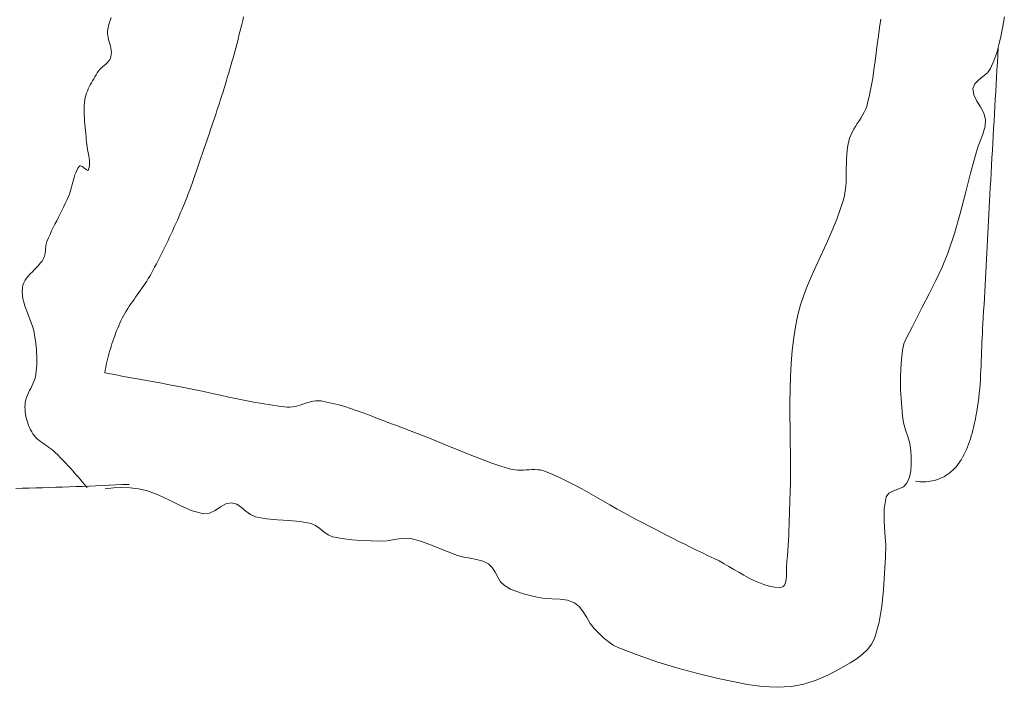
# Model space of a CAD drawing. Units: inches. Extents: x -15 to 423, y -713 to 71.
# Tile 13 of 24: x 333 to 357, y -341 to -324. Entities that reach past the tile are written whole.
import ezdxf

# ---------------------------------------------------------------- set-up
doc = ezdxf.new("R2010")
doc.units = ezdxf.units.IN
doc.header["$MEASUREMENT"] = 0
doc.layers.add('A-FURN', color=9, linetype='Continuous', lineweight=13)

# ---------------------------------------------------------------- blocks, each defined once
blk = doc.blocks.new('BED-DOUBLE')
for p, q in [((72.488, 18.091), (72.461, 18.02)), ((75.772, 18.106), (75.749, 18.013)), ((94.613, 17.825), (94.657, 18.111)), ((72.415, 17.876), (72.399, 17.803)), ((72.436, 17.949), (72.415, 17.876)), ((72.461, 18.02), (72.436, 17.949)), ((75.727, 17.92), (75.704, 17.827)), ((75.749, 18.013), (75.727, 17.92)), ((91.529, 17.634), (91.558, 17.844)), ((91.558, 17.844), (91.59, 18.053)), ((72.399, 17.803), (72.392, 17.751)), ((72.392, 17.751), (72.392, 17.698)), ((72.392, 17.698), (72.398, 17.646)), ((72.398, 17.646), (72.408, 17.593)), ((75.657, 17.642), (75.633, 17.549)), ((75.681, 17.735), (75.657, 17.642)), ((75.704, 17.827), (75.681, 17.735)), ((91.502, 17.424), (91.529, 17.634)), ((94.524, 17.415), (94.571, 17.62)), ((94.571, 17.62), (94.613, 17.825)), ((72.408, 17.593), (72.421, 17.54)), ((72.421, 17.54), (72.435, 17.487)), ((72.435, 17.487), (72.45, 17.434)), ((72.45, 17.434), (72.464, 17.382)), ((72.464, 17.382), (72.476, 17.329)), ((75.584, 17.364), (75.559, 17.272)), ((75.609, 17.457), (75.584, 17.364)), ((75.633, 17.549), (75.609, 17.457)), ((91.476, 17.214), (91.502, 17.424)), ((94.468, 17.212), (94.524, 17.415)), ((72.479, 17.121), (72.467, 17.083)), ((72.476, 17.329), (72.485, 17.276)), ((72.488, 17.172), (72.479, 17.121)), ((72.485, 17.276), (72.489, 17.224)), ((72.489, 17.224), (72.488, 17.172)), ((75.534, 17.179), (75.509, 17.087)), ((75.559, 17.272), (75.534, 17.179)), ((91.449, 17.004), (91.476, 17.214)), ((94.4, 17.014), (94.468, 17.212)), ((94.483, 16.977), (94.494, 17.16)), ((94.494, 17.16), (94.504, 17.342)), ((72.28, 16.872), (72.248, 16.844)), ((72.312, 16.899), (72.28, 16.872)), ((72.344, 16.927), (72.312, 16.899)), ((72.374, 16.955), (72.344, 16.927)), ((72.402, 16.984), (72.374, 16.955)), ((72.428, 17.015), (72.402, 16.984)), ((72.45, 17.048), (72.428, 17.015)), ((72.467, 17.083), (72.45, 17.048)), ((75.457, 16.903), (75.431, 16.811)), ((75.483, 16.995), (75.457, 16.903)), ((75.509, 17.087), (75.483, 16.995)), ((91.421, 16.794), (91.449, 17.004)), ((94.317, 16.822), (94.4, 17.014)), ((94.473, 16.795), (94.483, 16.977)), ((72.08, 16.623), (72.05, 16.573)), ((72.11, 16.672), (72.08, 16.623)), ((72.139, 16.721), (72.11, 16.672)), ((72.162, 16.754), (72.139, 16.721)), ((72.188, 16.785), (72.162, 16.754)), ((72.217, 16.815), (72.188, 16.785)), ((72.248, 16.844), (72.217, 16.815)), ((75.376, 16.625), (75.348, 16.53)), ((75.404, 16.719), (75.376, 16.625)), ((75.431, 16.811), (75.404, 16.719)), ((91.389, 16.585), (91.421, 16.794)), ((94.013, 16.539), (94.126, 16.626)), ((94.126, 16.626), (94.236, 16.716)), ((94.236, 16.716), (94.317, 16.822)), ((94.463, 16.612), (94.473, 16.795)), ((71.965, 16.422), (71.94, 16.371)), ((71.993, 16.473), (71.965, 16.422)), ((72.021, 16.523), (71.993, 16.473)), ((72.05, 16.573), (72.021, 16.523)), ((75.32, 16.436), (75.291, 16.342)), ((75.348, 16.53), (75.32, 16.436)), ((91.353, 16.376), (91.389, 16.585)), ((93.877, 16.327), (93.922, 16.444)), ((93.922, 16.444), (94.013, 16.539)), ((94.442, 16.248), (94.452, 16.43)), ((94.452, 16.43), (94.463, 16.612)), ((71.856, 16.159), (71.842, 16.104)), ((71.874, 16.213), (71.856, 16.159)), ((71.893, 16.266), (71.874, 16.213)), ((71.915, 16.319), (71.893, 16.266)), ((71.94, 16.371), (71.915, 16.319)), ((75.232, 16.155), (75.202, 16.061)), ((75.262, 16.248), (75.232, 16.155)), ((75.291, 16.342), (75.262, 16.248)), ((91.264, 15.963), (91.312, 16.169)), ((91.312, 16.169), (91.353, 16.376)), ((93.898, 16.169), (93.877, 16.327)), ((93.971, 16.019), (93.898, 16.169)), ((94.432, 16.065), (94.442, 16.248)), ((71.815, 15.897), (71.812, 15.821)), ((71.821, 15.972), (71.815, 15.897)), ((71.831, 16.048), (71.821, 15.972)), ((71.842, 16.104), (71.831, 16.048)), ((75.172, 15.967), (75.141, 15.874)), ((75.202, 16.061), (75.172, 15.967)), ((91.241, 15.886), (91.264, 15.963)), ((94.065, 15.871), (93.971, 16.019)), ((94.421, 15.883), (94.432, 16.065)), ((71.812, 15.821), (71.812, 15.745)), ((71.812, 15.745), (71.814, 15.668)), ((71.814, 15.668), (71.819, 15.592)), ((75.079, 15.687), (75.048, 15.594)), ((75.11, 15.78), (75.079, 15.687)), ((75.141, 15.874), (75.11, 15.78)), ((91.095, 15.597), (91.137, 15.668)), ((91.137, 15.668), (91.176, 15.739)), ((91.176, 15.739), (91.211, 15.812)), ((91.211, 15.812), (91.241, 15.886)), ((94.149, 15.721), (94.065, 15.871)), ((94.189, 15.562), (94.149, 15.721)), ((94.401, 15.518), (94.411, 15.7)), ((94.411, 15.7), (94.421, 15.883)), ((71.819, 15.592), (71.825, 15.515)), ((71.825, 15.515), (71.832, 15.439)), ((71.832, 15.439), (71.839, 15.362)), ((74.985, 15.407), (74.954, 15.314)), ((75.017, 15.5), (74.985, 15.407)), ((75.048, 15.594), (75.017, 15.5)), ((90.963, 15.389), (91.007, 15.458)), ((91.007, 15.458), (91.051, 15.528)), ((91.051, 15.528), (91.095, 15.597)), ((94.177, 15.392), (94.189, 15.562)), ((94.391, 15.335), (94.401, 15.518)), ((71.839, 15.362), (71.847, 15.285)), ((71.847, 15.285), (71.854, 15.209)), ((71.854, 15.209), (71.86, 15.132)), ((74.922, 15.221), (74.89, 15.128)), ((74.954, 15.314), (74.922, 15.221)), ((90.817, 15.1), (90.847, 15.175)), ((90.847, 15.175), (90.882, 15.247)), ((90.882, 15.247), (90.921, 15.319)), ((90.921, 15.319), (90.963, 15.389)), ((94.075, 15.061), (94.135, 15.225)), ((94.135, 15.225), (94.177, 15.392)), ((94.38, 15.153), (94.391, 15.335)), ((71.86, 15.132), (71.865, 15.056)), ((71.865, 15.056), (71.87, 14.999)), ((71.87, 14.999), (71.877, 14.942)), ((71.877, 14.942), (71.887, 14.884)), ((74.827, 14.942), (74.795, 14.849)), ((74.859, 15.035), (74.827, 14.942)), ((74.89, 15.128), (74.859, 15.035)), ((90.755, 14.802), (90.771, 14.913)), ((90.771, 14.913), (90.794, 15.023)), ((90.794, 15.023), (90.817, 15.1)), ((94.01, 14.897), (94.075, 15.061)), ((94.36, 14.788), (94.37, 14.971)), ((94.37, 14.971), (94.38, 15.153)), ((71.887, 14.884), (71.897, 14.827)), ((71.897, 14.827), (71.908, 14.769)), ((71.908, 14.769), (71.919, 14.712)), ((71.919, 14.712), (71.928, 14.654)), ((74.746, 14.703), (74.721, 14.63)), ((74.77, 14.776), (74.746, 14.703)), ((74.795, 14.849), (74.77, 14.776)), ((90.738, 14.577), (90.744, 14.69)), ((90.744, 14.69), (90.755, 14.802)), ((93.82, 14.232), (93.955, 14.732)), ((93.955, 14.732), (94.01, 14.897)), ((94.35, 14.606), (94.36, 14.788)), ((71.928, 14.654), (71.936, 14.597)), ((71.936, 14.597), (71.942, 14.54)), ((71.943, 14.427), (71.937, 14.371)), ((71.942, 14.54), (71.944, 14.484)), ((71.944, 14.484), (71.943, 14.427)), ((74.672, 14.485), (74.647, 14.412)), ((74.697, 14.557), (74.672, 14.485)), ((74.721, 14.63), (74.697, 14.557)), ((90.734, 14.351), (90.735, 14.464)), ((90.735, 14.464), (90.738, 14.577)), ((94.329, 14.241), (94.34, 14.423)), ((94.34, 14.423), (94.35, 14.606)), ((71.583, 14.184), (71.563, 14.125)), ((71.605, 14.241), (71.583, 14.184)), ((71.63, 14.296), (71.605, 14.241)), ((71.66, 14.349), (71.63, 14.296)), ((71.694, 14.399), (71.66, 14.349)), ((71.707, 14.41), (71.694, 14.399)), ((71.724, 14.411), (71.707, 14.41)), ((71.743, 14.405), (71.724, 14.411)), ((71.764, 14.394), (71.743, 14.405)), ((71.786, 14.379), (71.764, 14.394)), ((71.809, 14.361), (71.786, 14.379)), ((71.831, 14.344), (71.809, 14.361)), ((71.853, 14.327), (71.831, 14.344)), ((71.873, 14.313), (71.853, 14.327)), ((71.891, 14.303), (71.873, 14.313)), ((71.907, 14.299), (71.891, 14.303)), ((71.918, 14.303), (71.907, 14.299)), ((71.925, 14.316), (71.918, 14.303)), ((71.937, 14.371), (71.925, 14.316)), ((74.573, 14.194), (74.547, 14.121)), ((74.598, 14.266), (74.573, 14.194)), ((74.623, 14.339), (74.598, 14.266)), ((74.647, 14.412), (74.623, 14.339)), ((90.732, 14.124), (90.734, 14.237)), ((90.734, 14.237), (90.734, 14.351)), ((93.691, 13.73), (93.82, 14.232)), ((94.319, 14.058), (94.329, 14.241)), ((71.515, 13.945), (71.499, 13.884)), ((71.53, 14.005), (71.515, 13.945)), ((71.546, 14.066), (71.53, 14.005)), ((71.563, 14.125), (71.546, 14.066)), ((74.496, 13.976), (74.47, 13.904)), ((74.522, 14.049), (74.496, 13.976)), ((74.547, 14.121), (74.522, 14.049)), ((90.72, 13.898), (90.728, 14.011)), ((90.728, 14.011), (90.732, 14.124)), ((94.309, 13.876), (94.319, 14.058)), ((71.446, 13.705), (71.423, 13.648)), ((71.465, 13.764), (71.446, 13.705)), ((71.483, 13.824), (71.465, 13.764)), ((71.499, 13.884), (71.483, 13.824)), ((74.389, 13.688), (74.361, 13.617)), ((74.416, 13.76), (74.389, 13.688)), ((74.443, 13.832), (74.416, 13.76)), ((74.47, 13.904), (74.443, 13.832)), ((90.688, 13.677), (90.707, 13.787)), ((90.707, 13.787), (90.72, 13.898)), ((93.559, 13.23), (93.691, 13.73)), ((94.29, 13.533), (94.299, 13.693)), ((94.299, 13.693), (94.309, 13.876)), ((71.344, 13.475), (71.303, 13.389)), ((71.385, 13.561), (71.344, 13.475)), ((71.423, 13.648), (71.385, 13.561)), ((74.304, 13.474), (74.274, 13.404)), ((74.333, 13.546), (74.304, 13.474)), ((74.361, 13.617), (74.333, 13.546)), ((90.584, 13.325), (90.662, 13.568)), ((90.662, 13.568), (90.688, 13.677)), ((94.281, 13.373), (94.29, 13.533)), ((71.218, 13.219), (71.175, 13.135)), ((71.261, 13.304), (71.218, 13.219)), ((71.303, 13.389), (71.261, 13.304)), ((74.201, 13.233), (74.164, 13.148)), ((74.238, 13.318), (74.201, 13.233)), ((74.274, 13.404), (74.238, 13.318)), ((90.497, 13.085), (90.584, 13.325)), ((93.416, 12.733), (93.559, 13.23)), ((94.264, 13.053), (94.273, 13.213)), ((94.273, 13.213), (94.281, 13.373)), ((71.089, 12.965), (71.047, 12.88)), ((71.132, 13.05), (71.089, 12.965)), ((71.175, 13.135), (71.132, 13.05)), ((74.089, 12.979), (74.051, 12.894)), ((74.127, 13.064), (74.089, 12.979)), ((74.164, 13.148), (74.127, 13.064)), ((90.4, 12.848), (90.497, 13.085)), ((94.256, 12.893), (94.264, 13.053)), ((71.006, 12.794), (70.966, 12.708)), ((71.047, 12.88), (71.006, 12.794)), ((73.974, 12.726), (73.935, 12.642)), ((74.013, 12.81), (73.974, 12.726)), ((74.051, 12.894), (74.013, 12.81)), ((90.297, 12.612), (90.4, 12.848)), ((93.253, 12.242), (93.416, 12.733)), ((94.239, 12.572), (94.248, 12.733)), ((94.248, 12.733), (94.256, 12.893)), ((70.871, 12.47), (70.865, 12.437)), ((70.88, 12.502), (70.871, 12.47)), ((70.891, 12.534), (70.88, 12.502)), ((70.927, 12.621), (70.891, 12.534)), ((70.966, 12.708), (70.927, 12.621)), ((73.855, 12.474), (73.815, 12.391)), ((73.895, 12.558), (73.855, 12.474)), ((73.935, 12.642), (73.895, 12.558)), ((90.191, 12.378), (90.297, 12.612)), ((94.231, 12.412), (94.239, 12.572)), ((70.842, 12.235), (70.836, 12.202)), ((70.846, 12.268), (70.842, 12.235)), ((70.85, 12.302), (70.846, 12.268)), ((70.853, 12.336), (70.85, 12.302)), ((70.856, 12.37), (70.853, 12.336)), ((70.86, 12.403), (70.856, 12.37)), ((70.865, 12.437), (70.86, 12.403)), ((73.733, 12.225), (73.691, 12.142)), ((73.774, 12.308), (73.733, 12.225)), ((73.815, 12.391), (73.774, 12.308)), ((90.083, 12.145), (90.191, 12.378)), ((93.115, 11.899), (93.253, 12.242)), ((94.214, 12.092), (94.223, 12.252)), ((94.223, 12.252), (94.231, 12.412)), ((70.725, 11.993), (70.679, 11.939)), ((70.767, 12.049), (70.725, 11.993)), ((70.802, 12.108), (70.767, 12.049)), ((70.816, 12.138), (70.802, 12.108)), ((70.827, 12.17), (70.816, 12.138)), ((70.836, 12.202), (70.827, 12.17)), ((73.606, 11.977), (73.563, 11.895)), ((73.649, 12.06), (73.606, 11.977)), ((73.691, 12.142), (73.649, 12.06)), ((89.975, 11.911), (90.083, 12.145)), ((94.206, 11.932), (94.214, 12.092)), ((70.527, 11.783), (70.477, 11.732)), ((70.578, 11.835), (70.527, 11.783)), ((70.629, 11.886), (70.578, 11.835)), ((70.679, 11.939), (70.629, 11.886)), ((73.519, 11.814), (73.475, 11.732)), ((73.563, 11.895), (73.519, 11.814)), ((89.871, 11.676), (89.975, 11.911)), ((92.957, 11.564), (93.115, 11.899)), ((94.189, 11.612), (94.197, 11.772)), ((94.197, 11.772), (94.206, 11.932)), ((70.316, 11.511), (70.293, 11.449)), ((70.347, 11.57), (70.316, 11.511)), ((70.385, 11.626), (70.347, 11.57)), ((70.429, 11.68), (70.385, 11.626)), ((70.477, 11.732), (70.429, 11.68)), ((73.331, 11.495), (73.293, 11.438)), ((73.369, 11.553), (73.331, 11.495)), ((73.406, 11.612), (73.369, 11.553)), ((73.441, 11.672), (73.406, 11.612)), ((73.475, 11.732), (73.441, 11.672)), ((89.772, 11.441), (89.871, 11.676)), ((92.788, 11.233), (92.957, 11.564)), ((94.18, 11.451), (94.189, 11.612)), ((70.279, 11.383), (70.274, 11.292)), ((70.274, 11.292), (70.28, 11.202)), ((70.293, 11.449), (70.279, 11.383)), ((73.173, 11.267), (73.132, 11.21)), ((73.213, 11.323), (73.173, 11.267)), ((73.253, 11.38), (73.213, 11.323)), ((73.293, 11.438), (73.253, 11.38)), ((89.681, 11.202), (89.772, 11.441)), ((94.162, 11.131), (94.171, 11.291)), ((94.171, 11.291), (94.18, 11.451)), ((70.28, 11.202), (70.294, 11.113)), ((70.294, 11.113), (70.315, 11.025)), ((70.315, 11.025), (70.342, 10.936)), ((73.012, 11.04), (72.972, 10.983)), ((73.052, 11.097), (73.012, 11.04)), ((73.092, 11.153), (73.052, 11.097)), ((73.132, 11.21), (73.092, 11.153)), ((89.6, 10.961), (89.681, 11.202)), ((92.618, 10.903), (92.788, 11.233)), ((94.153, 10.971), (94.162, 11.131)), ((70.342, 10.936), (70.373, 10.849)), ((70.373, 10.849), (70.407, 10.761)), ((70.407, 10.761), (70.442, 10.673)), ((72.859, 10.808), (72.824, 10.749)), ((72.896, 10.867), (72.859, 10.808)), ((72.934, 10.925), (72.896, 10.867)), ((72.972, 10.983), (72.934, 10.925)), ((89.532, 10.717), (89.6, 10.961)), ((92.454, 10.571), (92.618, 10.903)), ((94.134, 10.651), (94.143, 10.811)), ((94.143, 10.811), (94.153, 10.971)), ((70.442, 10.673), (70.477, 10.585)), ((70.477, 10.585), (70.51, 10.497)), ((72.728, 10.565), (72.7, 10.503)), ((72.758, 10.627), (72.728, 10.565)), ((72.79, 10.688), (72.758, 10.627)), ((72.824, 10.749), (72.79, 10.688)), ((89.478, 10.468), (89.532, 10.717)), ((92.38, 10.427), (92.454, 10.571)), ((94.124, 10.491), (94.134, 10.651)), ((70.51, 10.497), (70.539, 10.408)), ((70.539, 10.408), (70.564, 10.319)), ((70.564, 10.319), (70.582, 10.229)), ((72.62, 10.316), (72.595, 10.253)), ((72.646, 10.379), (72.62, 10.316)), ((72.672, 10.441), (72.646, 10.379)), ((72.7, 10.503), (72.672, 10.441)), ((89.428, 10.15), (89.478, 10.468)), ((92.224, 10.142), (92.3, 10.285)), ((92.3, 10.285), (92.38, 10.427)), ((94.111, 10.262), (94.117, 10.376)), ((94.117, 10.376), (94.124, 10.491)), ((70.582, 10.229), (70.593, 10.153)), ((70.593, 10.153), (70.604, 10.077)), ((70.604, 10.077), (70.613, 10.001)), ((72.526, 10.062), (72.504, 9.997)), ((72.548, 10.126), (72.526, 10.062)), ((72.571, 10.19), (72.548, 10.126)), ((72.595, 10.253), (72.571, 10.19)), ((89.39, 9.83), (89.428, 10.15)), ((92.163, 9.994), (92.224, 10.142)), ((94.097, 9.917), (94.101, 10.032)), ((94.101, 10.032), (94.106, 10.147)), ((94.106, 10.147), (94.111, 10.262)), ((70.613, 10.001), (70.621, 9.924)), ((70.621, 9.924), (70.628, 9.848)), ((70.628, 9.848), (70.633, 9.771)), ((72.445, 9.802), (72.427, 9.736)), ((72.464, 9.867), (72.445, 9.802)), ((72.484, 9.932), (72.464, 9.867)), ((72.504, 9.997), (72.484, 9.932)), ((89.363, 9.509), (89.39, 9.83)), ((92.092, 9.515), (92.125, 9.84)), ((92.125, 9.84), (92.163, 9.994)), ((94.089, 9.687), (94.093, 9.802)), ((94.093, 9.802), (94.097, 9.917)), ((70.633, 9.771), (70.636, 9.695)), ((70.636, 9.695), (70.638, 9.618)), ((70.638, 9.541), (70.636, 9.465)), ((70.638, 9.618), (70.638, 9.541)), ((72.379, 9.539), (72.364, 9.472)), ((72.394, 9.605), (72.379, 9.539)), ((72.41, 9.671), (72.394, 9.605)), ((72.427, 9.736), (72.41, 9.671)), ((94.08, 9.457), (94.085, 9.572)), ((94.085, 9.572), (94.089, 9.687)), ((70.625, 9.312), (70.616, 9.236)), ((70.631, 9.388), (70.625, 9.312)), ((70.636, 9.465), (70.631, 9.388)), ((72.339, 9.339), (72.327, 9.273)), ((72.351, 9.406), (72.339, 9.339)), ((72.364, 9.472), (72.351, 9.406)), ((89.346, 9.187), (89.363, 9.509)), ((92.079, 9.189), (92.092, 9.515)), ((94.069, 9.227), (94.075, 9.342)), ((94.075, 9.342), (94.08, 9.457)), ((70.566, 9.06), (70.541, 9.002)), ((70.588, 9.117), (70.566, 9.06)), ((70.604, 9.176), (70.588, 9.117)), ((70.616, 9.236), (70.604, 9.176)), ((72.327, 9.273), (72.469, 9.247)), ((72.469, 9.247), (72.61, 9.222)), ((72.61, 9.222), (72.751, 9.196)), ((72.751, 9.196), (72.893, 9.171)), ((72.893, 9.171), (73.034, 9.145)), ((73.034, 9.145), (73.176, 9.119)), ((73.176, 9.119), (73.317, 9.094)), ((73.317, 9.094), (73.459, 9.068)), ((73.459, 9.068), (73.6, 9.041)), ((89.337, 8.864), (89.346, 9.187)), ((92.083, 8.861), (92.079, 9.189)), ((94.054, 8.997), (94.062, 9.112)), ((94.062, 9.112), (94.069, 9.227)), ((70.458, 8.834), (70.43, 8.777)), ((70.486, 8.89), (70.458, 8.834)), ((70.514, 8.946), (70.486, 8.89)), ((70.541, 9.002), (70.514, 8.946)), ((73.6, 9.041), (73.741, 9.015)), ((73.741, 9.015), (73.883, 8.989)), ((73.883, 8.989), (74.024, 8.963)), ((74.024, 8.963), (74.165, 8.936)), ((74.165, 8.936), (74.372, 8.896)), ((74.372, 8.896), (74.578, 8.854)), ((74.578, 8.854), (74.784, 8.809)), ((74.784, 8.809), (74.991, 8.764)), ((89.334, 8.541), (89.337, 8.864)), ((92.1, 8.534), (92.083, 8.861)), ((94.034, 8.769), (94.045, 8.883)), ((94.045, 8.883), (94.054, 8.997)), ((70.365, 8.605), (70.352, 8.546)), ((70.383, 8.663), (70.365, 8.605)), ((70.405, 8.721), (70.383, 8.663)), ((70.43, 8.777), (70.405, 8.721)), ((74.991, 8.764), (75.196, 8.719)), ((75.196, 8.719), (75.402, 8.674)), ((75.402, 8.674), (75.609, 8.63)), ((75.609, 8.63), (75.815, 8.587)), ((75.815, 8.587), (76.022, 8.547)), ((77.371, 8.54), (77.436, 8.559)), ((77.436, 8.559), (77.5, 8.573)), ((77.5, 8.573), (77.564, 8.582)), ((77.564, 8.582), (77.629, 8.584)), ((77.629, 8.584), (77.694, 8.578)), ((77.694, 8.578), (77.842, 8.55)), ((94.007, 8.541), (94.021, 8.655)), ((94.021, 8.655), (94.034, 8.769)), ((70.345, 8.485), (70.344, 8.427)), ((70.344, 8.427), (70.345, 8.369)), ((70.352, 8.546), (70.345, 8.485)), ((70.345, 8.369), (70.35, 8.311)), ((70.35, 8.311), (70.357, 8.253)), ((76.022, 8.547), (76.229, 8.51)), ((76.229, 8.51), (76.437, 8.477)), ((76.437, 8.477), (76.645, 8.448)), ((76.645, 8.448), (76.854, 8.424)), ((76.854, 8.424), (76.919, 8.422)), ((76.919, 8.422), (76.984, 8.427)), ((76.984, 8.427), (77.049, 8.439)), ((77.049, 8.439), (77.114, 8.455)), ((77.114, 8.455), (77.178, 8.475)), ((77.178, 8.475), (77.243, 8.497)), ((77.243, 8.497), (77.307, 8.519)), ((77.307, 8.519), (77.371, 8.54)), ((77.842, 8.55), (77.989, 8.517)), ((77.989, 8.517), (78.136, 8.479)), ((78.136, 8.479), (78.281, 8.437)), ((78.281, 8.437), (78.425, 8.391)), ((78.425, 8.391), (78.568, 8.342)), ((78.568, 8.342), (78.711, 8.291)), ((89.335, 8.217), (89.334, 8.541)), ((92.125, 8.207), (92.1, 8.534)), ((93.951, 8.202), (93.972, 8.315)), ((93.972, 8.315), (93.991, 8.428)), ((93.991, 8.428), (94.007, 8.541)), ((70.357, 8.253), (70.368, 8.195)), ((70.368, 8.195), (70.381, 8.137)), ((70.381, 8.137), (70.396, 8.08)), ((70.396, 8.08), (70.415, 8.024)), ((78.711, 8.291), (78.854, 8.238)), ((78.854, 8.238), (78.996, 8.184)), ((78.996, 8.184), (79.138, 8.129)), ((79.138, 8.129), (79.28, 8.075)), ((79.28, 8.075), (79.422, 8.021)), ((89.338, 7.893), (89.335, 8.217)), ((92.154, 8.033), (92.125, 8.207)), ((93.923, 8.062), (93.937, 8.132)), ((93.937, 8.132), (93.951, 8.202)), ((70.415, 8.024), (70.435, 7.969)), ((70.435, 7.969), (70.458, 7.915)), ((70.458, 7.915), (70.484, 7.862)), ((70.484, 7.862), (70.511, 7.811)), ((79.422, 8.021), (79.564, 7.969)), ((79.564, 7.969), (79.781, 7.889)), ((79.781, 7.889), (79.997, 7.806)), ((89.343, 7.568), (89.338, 7.893)), ((92.204, 7.862), (92.154, 8.033)), ((92.261, 7.693), (92.204, 7.862)), ((93.856, 7.781), (93.874, 7.851)), ((93.874, 7.851), (93.891, 7.921)), ((93.891, 7.921), (93.907, 7.992)), ((93.907, 7.992), (93.923, 8.062)), ((70.511, 7.811), (70.541, 7.761)), ((70.541, 7.761), (70.573, 7.716)), ((70.573, 7.716), (70.608, 7.675)), ((70.608, 7.675), (70.647, 7.637)), ((70.647, 7.637), (70.689, 7.601)), ((70.689, 7.601), (70.733, 7.567)), ((79.997, 7.806), (80.213, 7.72)), ((80.213, 7.72), (80.428, 7.633)), ((80.428, 7.633), (80.642, 7.545)), ((92.309, 7.522), (92.261, 7.693)), ((93.793, 7.572), (93.815, 7.641)), ((93.815, 7.641), (93.836, 7.711)), ((93.836, 7.711), (93.856, 7.781)), ((70.733, 7.567), (70.778, 7.534)), ((70.778, 7.534), (70.825, 7.503)), ((70.825, 7.503), (70.872, 7.471)), ((70.872, 7.471), (70.919, 7.44)), ((70.919, 7.44), (70.965, 7.407)), ((70.965, 7.407), (71.01, 7.374)), ((71.01, 7.374), (71.053, 7.338)), ((71.053, 7.338), (71.093, 7.301)), ((80.642, 7.545), (80.857, 7.457)), ((80.857, 7.457), (81.071, 7.369)), ((81.071, 7.369), (81.286, 7.282)), ((89.347, 7.244), (89.343, 7.568)), ((92.337, 7.347), (92.309, 7.522)), ((92.346, 7.181), (92.337, 7.347)), ((93.686, 7.305), (93.715, 7.37)), ((93.715, 7.37), (93.743, 7.436)), ((93.743, 7.436), (93.769, 7.504)), ((93.769, 7.504), (93.793, 7.572)), ((71.093, 7.301), (71.158, 7.237)), ((71.158, 7.237), (71.222, 7.172)), ((71.222, 7.172), (71.285, 7.107)), ((71.285, 7.107), (71.348, 7.041)), ((81.286, 7.282), (81.502, 7.197)), ((81.502, 7.197), (81.718, 7.115)), ((81.718, 7.115), (81.936, 7.036)), ((89.349, 6.92), (89.347, 7.244)), ((92.348, 7.012), (92.346, 7.181)), ((93.546, 7.059), (93.584, 7.118)), ((93.584, 7.118), (93.62, 7.179)), ((93.62, 7.179), (93.654, 7.241)), ((93.654, 7.241), (93.686, 7.305)), ((71.348, 7.041), (71.41, 6.974)), ((71.41, 6.974), (71.472, 6.908)), ((71.472, 6.908), (71.533, 6.84)), ((81.936, 7.036), (82.155, 6.961)), ((82.155, 6.961), (82.375, 6.89)), ((82.375, 6.89), (82.442, 6.874)), ((82.442, 6.874), (82.51, 6.864)), ((82.51, 6.864), (82.579, 6.86)), ((82.579, 6.86), (82.648, 6.859)), ((82.648, 6.859), (82.719, 6.862)), ((82.719, 6.862), (82.789, 6.866)), ((82.789, 6.866), (82.86, 6.871)), ((82.86, 6.871), (82.93, 6.874)), ((82.93, 6.874), (83, 6.875)), ((83, 6.875), (83.069, 6.872)), ((83.069, 6.872), (83.136, 6.865)), ((83.136, 6.865), (83.203, 6.851)), ((83.203, 6.851), (83.268, 6.829)), ((89.346, 6.597), (89.349, 6.92)), ((92.3, 6.684), (92.334, 6.846)), ((92.334, 6.846), (92.348, 7.012)), ((93.341, 6.823), (93.379, 6.857)), ((93.379, 6.857), (93.414, 6.893)), ((93.414, 6.893), (93.461, 6.946)), ((93.461, 6.946), (93.505, 7.002)), ((93.505, 7.002), (93.546, 7.059)), ((71.533, 6.84), (71.594, 6.772)), ((71.594, 6.772), (71.654, 6.704)), ((71.654, 6.704), (71.713, 6.635)), ((71.713, 6.635), (71.772, 6.566)), ((83.268, 6.829), (83.452, 6.752)), ((83.452, 6.752), (83.634, 6.669)), ((83.634, 6.669), (83.814, 6.581)), ((92.239, 6.533), (92.3, 6.684)), ((92.869, 6.594), (92.921, 6.607)), ((92.921, 6.607), (92.972, 6.622)), ((92.972, 6.622), (93.023, 6.639)), ((93.023, 6.639), (93.072, 6.659)), ((93.072, 6.659), (93.121, 6.681)), ((93.121, 6.681), (93.168, 6.706)), ((93.168, 6.706), (93.214, 6.732)), ((93.214, 6.732), (93.258, 6.76)), ((93.258, 6.76), (93.301, 6.791)), ((93.301, 6.791), (93.341, 6.823)), ((70.12, 6.405), (70.285, 6.41)), ((70.285, 6.41), (70.45, 6.414)), ((70.45, 6.414), (70.616, 6.419)), ((70.616, 6.419), (70.781, 6.424)), ((70.781, 6.424), (70.947, 6.429)), ((70.947, 6.429), (71.112, 6.434)), ((71.112, 6.434), (71.277, 6.44)), ((71.277, 6.44), (71.443, 6.446)), ((71.443, 6.446), (71.608, 6.452)), ((71.608, 6.452), (71.773, 6.458)), ((71.772, 6.566), (71.831, 6.497)), ((71.773, 6.458), (71.939, 6.464)), ((71.831, 6.497), (71.888, 6.426)), ((71.939, 6.464), (72.104, 6.471)), ((72.104, 6.471), (72.269, 6.478)), ((72.269, 6.478), (72.434, 6.485)), ((72.335, 6.396), (72.54, 6.421)), ((72.434, 6.485), (72.6, 6.493)), ((72.54, 6.421), (72.747, 6.429)), ((72.6, 6.493), (72.765, 6.5)), ((72.747, 6.429), (72.955, 6.42)), ((72.765, 6.5), (72.93, 6.508)), ((72.955, 6.42), (73.161, 6.394)), ((73.161, 6.394), (73.364, 6.352)), ((83.814, 6.581), (83.992, 6.489)), ((83.992, 6.489), (84.169, 6.394)), ((84.169, 6.394), (84.344, 6.296)), ((89.337, 6.274), (89.346, 6.597)), ((91.903, 6.348), (92.034, 6.393)), ((92.034, 6.393), (92.155, 6.448)), ((92.155, 6.448), (92.239, 6.533)), ((92.454, 6.586), (92.504, 6.578)), ((92.504, 6.578), (92.555, 6.572)), ((92.555, 6.572), (92.606, 6.569)), ((92.606, 6.569), (92.659, 6.568)), ((92.659, 6.568), (92.711, 6.571)), ((92.711, 6.571), (92.764, 6.576)), ((92.764, 6.576), (92.816, 6.584)), ((92.816, 6.584), (92.869, 6.594)), ((73.364, 6.352), (73.654, 6.25)), ((73.654, 6.25), (73.933, 6.114)), ((73.933, 6.114), (74.21, 5.972)), ((84.344, 6.296), (84.519, 6.197)), ((84.519, 6.197), (84.693, 6.097)), ((89.329, 6.016), (89.333, 6.145)), ((89.333, 6.145), (89.337, 6.274)), ((91.675, 5.904), (91.726, 6.196)), ((91.726, 6.196), (91.792, 6.289)), ((91.792, 6.289), (91.903, 6.348)), ((74.21, 5.972), (74.493, 5.849)), ((75.064, 5.858), (75.197, 5.946)), ((75.197, 5.946), (75.332, 6.021)), ((75.332, 6.021), (75.475, 6.047)), ((75.475, 6.047), (75.603, 6.012)), ((75.603, 6.012), (75.719, 5.937)), ((75.719, 5.937), (75.83, 5.845)), ((84.693, 6.097), (84.867, 5.996)), ((84.867, 5.996), (85.042, 5.896)), ((85.042, 5.896), (85.217, 5.798)), ((89.322, 5.759), (89.325, 5.888)), ((89.325, 5.888), (89.329, 6.016)), ((91.671, 5.606), (91.675, 5.904)), ((74.493, 5.849), (74.788, 5.773)), ((74.788, 5.773), (74.929, 5.789)), ((74.929, 5.789), (75.064, 5.858)), ((75.83, 5.845), (75.944, 5.76)), ((75.944, 5.76), (76.069, 5.703)), ((76.069, 5.703), (76.341, 5.651)), ((76.341, 5.651), (76.617, 5.626)), ((76.617, 5.626), (76.896, 5.609)), ((85.217, 5.798), (85.393, 5.701)), ((85.393, 5.701), (85.57, 5.607)), ((89.314, 5.502), (89.318, 5.631)), ((89.318, 5.631), (89.322, 5.759)), ((76.896, 5.609), (77.173, 5.584)), ((77.173, 5.584), (77.445, 5.533)), ((77.445, 5.533), (77.558, 5.484)), ((77.558, 5.484), (77.662, 5.411)), ((77.662, 5.411), (77.763, 5.33)), ((85.57, 5.607), (85.714, 5.533)), ((85.714, 5.533), (85.858, 5.459)), ((85.858, 5.459), (86.002, 5.385)), ((86.002, 5.385), (86.146, 5.312)), ((89.31, 5.374), (89.314, 5.502)), ((91.692, 5.303), (91.671, 5.606)), ((77.763, 5.33), (77.867, 5.257)), ((77.867, 5.257), (77.981, 5.209)), ((77.981, 5.209), (78.217, 5.162)), ((78.217, 5.162), (78.457, 5.132)), ((79.332, 5.11), (79.48, 5.134)), ((79.48, 5.134), (79.629, 5.159)), ((79.629, 5.159), (79.777, 5.173)), ((79.777, 5.173), (79.923, 5.162)), ((79.923, 5.162), (80.161, 5.102)), ((86.146, 5.312), (86.29, 5.238)), ((86.29, 5.238), (86.435, 5.165)), ((86.435, 5.165), (86.579, 5.093)), ((89.298, 5.117), (89.304, 5.245)), ((89.304, 5.245), (89.31, 5.374)), ((91.713, 5), (91.692, 5.303)), ((78.457, 5.132), (78.699, 5.116)), ((78.699, 5.116), (78.941, 5.108)), ((78.941, 5.108), (79.183, 5.102)), ((79.183, 5.102), (79.332, 5.11)), ((80.161, 5.102), (80.392, 5.019)), ((80.392, 5.019), (80.62, 4.925)), ((80.62, 4.925), (80.848, 4.83)), ((86.579, 5.093), (86.724, 5.021)), ((86.724, 5.021), (86.869, 4.949)), ((86.869, 4.949), (87.014, 4.878)), ((89.281, 4.86), (89.29, 4.988)), ((89.29, 4.988), (89.298, 5.117)), ((91.709, 4.7), (91.713, 5)), ((80.848, 4.83), (81.079, 4.745)), ((81.079, 4.745), (81.235, 4.705)), ((81.235, 4.705), (81.396, 4.676)), ((81.396, 4.676), (81.555, 4.645)), ((81.555, 4.645), (81.709, 4.601)), ((87.014, 4.878), (87.16, 4.807)), ((87.16, 4.807), (87.306, 4.737)), ((87.306, 4.737), (87.452, 4.667)), ((87.452, 4.667), (87.575, 4.606)), ((89.258, 4.604), (89.27, 4.732)), ((89.27, 4.732), (89.281, 4.86)), ((91.681, 4.297), (91.709, 4.7)), ((81.709, 4.601), (81.851, 4.532)), ((81.851, 4.532), (81.946, 4.442)), ((81.946, 4.442), (82.018, 4.328)), ((87.575, 4.606), (87.698, 4.539)), ((87.698, 4.539), (87.82, 4.469)), ((87.82, 4.469), (87.942, 4.397)), ((89.252, 4.487), (89.254, 4.549)), ((89.252, 4.422), (89.252, 4.487)), ((89.253, 4.355), (89.252, 4.422)), ((89.254, 4.549), (89.258, 4.604)), ((82.018, 4.328), (82.082, 4.205)), ((82.082, 4.205), (82.153, 4.09)), ((87.942, 4.397), (88.064, 4.325)), ((88.064, 4.325), (88.186, 4.254)), ((88.186, 4.254), (88.309, 4.187)), ((88.309, 4.187), (88.434, 4.125)), ((89.235, 4.099), (89.244, 4.157)), ((89.244, 4.157), (89.25, 4.221)), ((89.25, 4.221), (89.252, 4.287)), ((89.252, 4.287), (89.253, 4.355)), ((91.655, 3.892), (91.681, 4.297)), ((82.153, 4.09), (82.246, 3.997)), ((82.246, 3.997), (82.395, 3.911)), ((82.395, 3.911), (82.553, 3.845)), ((88.434, 4.125), (88.56, 4.069)), ((88.56, 4.069), (88.688, 4.022)), ((88.688, 4.022), (88.818, 3.985)), ((88.818, 3.985), (88.951, 3.96)), ((88.951, 3.96), (89.086, 3.947)), ((89.086, 3.947), (89.133, 3.953)), ((89.133, 3.953), (89.17, 3.973)), ((89.17, 3.973), (89.199, 4.005)), ((89.199, 4.005), (89.22, 4.048)), ((89.22, 4.048), (89.235, 4.099)), ((82.553, 3.845), (82.719, 3.791)), ((82.719, 3.791), (82.887, 3.747)), ((82.887, 3.747), (83.056, 3.706)), ((83.056, 3.706), (83.243, 3.677)), ((83.243, 3.677), (83.435, 3.667)), ((83.435, 3.667), (83.627, 3.658)), ((91.616, 3.489), (91.655, 3.892)), ((83.627, 3.658), (83.812, 3.631)), ((83.812, 3.631), (83.985, 3.566)), ((83.985, 3.566), (84.108, 3.47)), ((84.108, 3.47), (84.205, 3.343)), ((91.551, 3.092), (91.616, 3.489)), ((84.205, 3.343), (84.289, 3.201)), ((84.289, 3.201), (84.374, 3.059)), ((84.374, 3.059), (84.475, 2.933)), ((91.446, 2.705), (91.551, 3.092)), ((84.475, 2.933), (84.585, 2.821)), ((84.585, 2.821), (84.699, 2.711)), ((84.699, 2.711), (84.819, 2.609)), ((91.371, 2.547), (91.446, 2.705)), ((84.819, 2.609), (84.947, 2.521)), ((84.947, 2.521), (85.085, 2.451)), ((85.085, 2.451), (85.568, 2.267)), ((91.262, 2.407), (91.371, 2.547)), ((85.568, 2.267), (86.057, 2.099)), ((90.981, 2.174), (91.129, 2.283)), ((91.129, 2.283), (91.262, 2.407)), ((86.057, 2.099), (86.552, 1.947)), ((90.554, 1.922), (90.829, 2.078)), ((90.829, 2.078), (90.981, 2.174)), ((86.552, 1.947), (87.051, 1.812)), ((87.051, 1.812), (87.554, 1.691)), ((89.982, 1.649), (90.272, 1.775)), ((90.272, 1.775), (90.554, 1.922)), ((87.554, 1.691), (87.914, 1.613)), ((87.914, 1.613), (88.278, 1.543)), ((88.278, 1.543), (88.645, 1.493)), ((88.645, 1.493), (89.011, 1.472)), ((89.011, 1.472), (89.376, 1.492)), ((89.376, 1.492), (89.683, 1.551)), ((89.683, 1.551), (89.982, 1.649))]:
    blk.add_line(p, q)

msp = doc.modelspace()

# ---------------------------------------------------------------- block references
at = {"layer": 'A-FURN'}
msp.add_blockref('BED-DOUBLE', (262.678, -342.175), dxfattribs=at)

doc.saveas('drawing.dxf')
